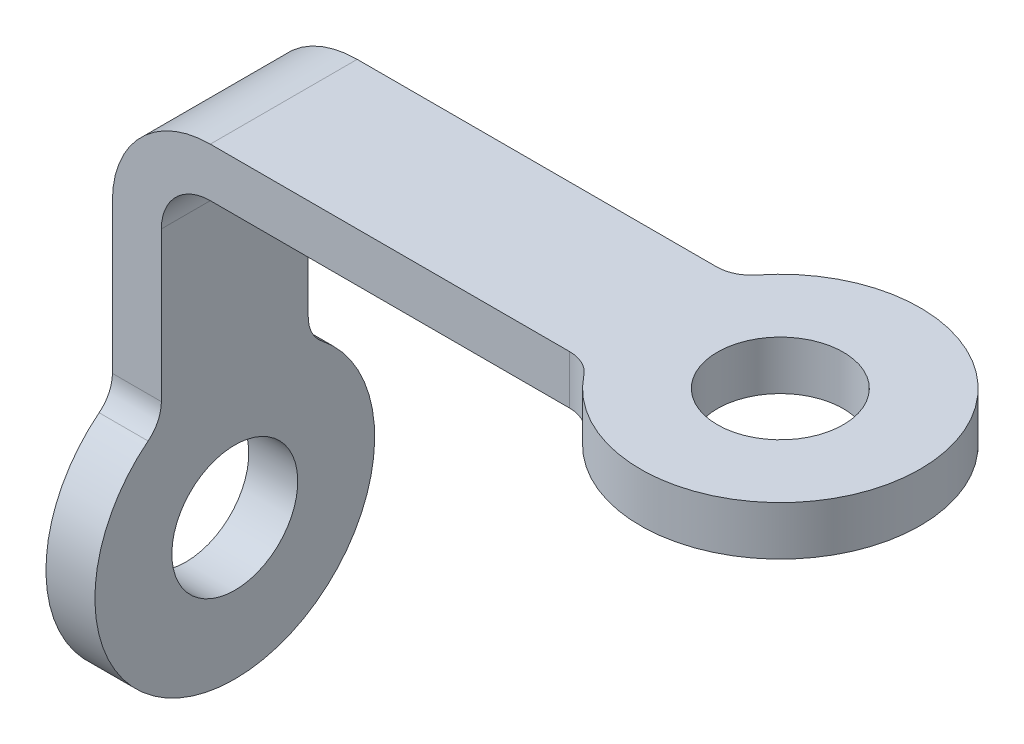
ISO-10303-21;
HEADER;
FILE_DESCRIPTION(('STEP AP214'),'2;1');
FILE_NAME('part.step','',(''),(''),'','','');
FILE_SCHEMA(('AUTOMOTIVE_DESIGN { 1 0 10303 214 1 1 1 1 }'));
ENDSEC;
DATA;
#1=APPLICATION_CONTEXT('core data for automotive mechanical design processes');
#2=APPLICATION_PROTOCOL_DEFINITION('international standard','automotive_design',2000,#1);
#3=PRODUCT_CONTEXT('',#1,'mechanical');
#4=PRODUCT('Part','Part','',(#3));
#5=PRODUCT_RELATED_PRODUCT_CATEGORY('part','',(#4));
#6=PRODUCT_DEFINITION_FORMATION('','',#4);
#7=PRODUCT_DEFINITION_CONTEXT('part definition',#1,'design');
#8=PRODUCT_DEFINITION('design','',#6,#7);
#9=PRODUCT_DEFINITION_SHAPE('','',#8);
#10=(LENGTH_UNIT() NAMED_UNIT(*) SI_UNIT(.MILLI.,.METRE.));
#11=(NAMED_UNIT(*) PLANE_ANGLE_UNIT() SI_UNIT($,.RADIAN.));
#12=(NAMED_UNIT(*) SI_UNIT($,.STERADIAN.) SOLID_ANGLE_UNIT());
#13=UNCERTAINTY_MEASURE_WITH_UNIT(LENGTH_MEASURE(1.E-05),#10,'distance_accuracy_value','');
#14=(GEOMETRIC_REPRESENTATION_CONTEXT(3) GLOBAL_UNCERTAINTY_ASSIGNED_CONTEXT((#13)) GLOBAL_UNIT_ASSIGNED_CONTEXT((#10,
#11,#12)) REPRESENTATION_CONTEXT('',''));
#15=CARTESIAN_POINT('',(0.,0.,0.));
#16=DIRECTION('',(0.,0.,1.));
#17=DIRECTION('',(1.,0.,0.));
#18=AXIS2_PLACEMENT_3D('',#15,#16,#17);
#19=CARTESIAN_POINT('',(85.,0.,10.5));
#20=DIRECTION('',(0.,-1.,0.));
#21=DIRECTION('',(0.,0.,-1.));
#22=AXIS2_PLACEMENT_3D('',#19,#20,#21);
#23=PLANE('',#22);
#24=CARTESIAN_POINT('',(85.,0.,0.));
#25=DIRECTION('',(0.,1.,0.));
#26=DIRECTION('',(0.,0.,1.));
#27=AXIS2_PLACEMENT_3D('',#24,#25,#26);
#28=CIRCLE('',#27,9.);
#29=CARTESIAN_POINT('',(85.,0.,9.));
#30=VERTEX_POINT('',#29);
#31=EDGE_CURVE('E253',#30,#30,#28,.T.);
#32=ORIENTED_EDGE('',*,*,#31,.F.);
#33=EDGE_LOOP('',(#32));
#34=FACE_BOUND('',#33,.T.);
#35=CARTESIAN_POINT('',(85.,0.,0.));
#36=DIRECTION('',(0.,1.,0.));
#37=DIRECTION('',(0.,0.,1.));
#38=AXIS2_PLACEMENT_3D('',#35,#36,#37);
#39=CIRCLE('',#38,20.);
#40=CARTESIAN_POINT('',(69.3079638032536,0.,12.4));
#41=VERTEX_POINT('',#40);
#42=CARTESIAN_POINT('',(69.3079638032536,0.,-12.4));
#43=VERTEX_POINT('',#42);
#44=EDGE_CURVE('E234',#41,#43,#39,.T.);
#45=ORIENTED_EDGE('',*,*,#44,.T.);
#46=CARTESIAN_POINT('',(65.384954754067,0.,-15.5));
#47=DIRECTION('',(0.,-1.,0.));
#48=DIRECTION('',(0.,0.,-1.));
#49=AXIS2_PLACEMENT_3D('',#46,#47,#48);
#50=CIRCLE('',#49,5.);
#51=CARTESIAN_POINT('',(65.384954754067,0.,-10.5));
#52=VERTEX_POINT('',#51);
#53=EDGE_CURVE('E230',#43,#52,#50,.T.);
#54=ORIENTED_EDGE('',*,*,#53,.T.);
#55=DIRECTION('',(-1.,0.,0.));
#56=VECTOR('',#55,1.);
#57=CARTESIAN_POINT('',(85.,0.,-10.5));
#58=LINE('',#57,#56);
#59=CARTESIAN_POINT('',(14.,0.,-10.5));
#60=VERTEX_POINT('',#59);
#61=EDGE_CURVE('E179',#52,#60,#58,.T.);
#62=ORIENTED_EDGE('',*,*,#61,.T.);
#63=DIRECTION('',(0.,0.,-1.));
#64=VECTOR('',#63,1.);
#65=CARTESIAN_POINT('',(14.,0.,10.5));
#66=LINE('',#65,#64);
#67=CARTESIAN_POINT('',(14.,0.,10.5));
#68=VERTEX_POINT('',#67);
#69=EDGE_CURVE('E159',#60,#68,#66,.F.);
#70=ORIENTED_EDGE('',*,*,#69,.T.);
#71=DIRECTION('',(-1.,0.,0.));
#72=VECTOR('',#71,1.);
#73=CARTESIAN_POINT('',(85.,0.,10.5));
#74=LINE('',#73,#72);
#75=CARTESIAN_POINT('',(65.384954754067,0.,10.5));
#76=VERTEX_POINT('',#75);
#77=EDGE_CURVE('E189',#76,#68,#74,.T.);
#78=ORIENTED_EDGE('',*,*,#77,.F.);
#79=CARTESIAN_POINT('',(65.384954754067,0.,15.5));
#80=DIRECTION('',(0.,-1.,0.));
#81=DIRECTION('',(0.,0.,-1.));
#82=AXIS2_PLACEMENT_3D('',#79,#80,#81);
#83=CIRCLE('',#82,5.);
#84=EDGE_CURVE('E69',#76,#41,#83,.T.);
#85=ORIENTED_EDGE('',*,*,#84,.T.);
#86=EDGE_LOOP('',(#45,#54,#62,#70,#78,#85));
#87=FACE_BOUND('',#86,.T.);
#88=ADVANCED_FACE('F65',(#34,#87),#23,.F.);
#89=CARTESIAN_POINT('',(0.,0.,10.5));
#90=DIRECTION('',(1.,0.,0.));
#91=DIRECTION('',(0.,1.,0.));
#92=AXIS2_PLACEMENT_3D('',#89,#90,#91);
#93=PLANE('',#92);
#94=DIRECTION('',(0.,-1.,0.));
#95=VECTOR('',#94,1.);
#96=CARTESIAN_POINT('',(0.,0.,10.5));
#97=LINE('',#96,#95);
#98=CARTESIAN_POINT('',(0.,-14.,10.5));
#99=VERTEX_POINT('',#98);
#100=CARTESIAN_POINT('',(0.,-35.384954754067,10.5));
#101=VERTEX_POINT('',#100);
#102=EDGE_CURVE('E171',#99,#101,#97,.T.);
#103=ORIENTED_EDGE('',*,*,#102,.F.);
#104=DIRECTION('',(0.,0.,-1.));
#105=VECTOR('',#104,1.);
#106=CARTESIAN_POINT('',(0.,-14.,10.5));
#107=LINE('',#106,#105);
#108=CARTESIAN_POINT('',(0.,-14.,-10.5));
#109=VERTEX_POINT('',#108);
#110=EDGE_CURVE('E160',#99,#109,#107,.T.);
#111=ORIENTED_EDGE('',*,*,#110,.T.);
#112=DIRECTION('',(0.,-1.,0.));
#113=VECTOR('',#112,1.);
#114=CARTESIAN_POINT('',(0.,0.,-10.5));
#115=LINE('',#114,#113);
#116=CARTESIAN_POINT('',(0.,-35.384954754067,-10.5));
#117=VERTEX_POINT('',#116);
#118=EDGE_CURVE('E169',#109,#117,#115,.T.);
#119=ORIENTED_EDGE('',*,*,#118,.T.);
#120=CARTESIAN_POINT('',(0.,-35.384954754067,-15.5));
#121=DIRECTION('',(1.,0.,0.));
#122=DIRECTION('',(0.,1.,0.));
#123=AXIS2_PLACEMENT_3D('',#120,#121,#122);
#124=CIRCLE('',#123,5.);
#125=CARTESIAN_POINT('',(0.,-39.3079638032536,-12.4));
#126=VERTEX_POINT('',#125);
#127=EDGE_CURVE('E223',#117,#126,#124,.T.);
#128=ORIENTED_EDGE('',*,*,#127,.T.);
#129=CARTESIAN_POINT('',(0.,-55.,0.));
#130=DIRECTION('',(-1.,0.,0.));
#131=DIRECTION('',(0.,-1.,0.));
#132=AXIS2_PLACEMENT_3D('',#129,#130,#131);
#133=CIRCLE('',#132,20.);
#134=CARTESIAN_POINT('',(0.,-39.3079638032536,12.4));
#135=VERTEX_POINT('',#134);
#136=EDGE_CURVE('E263',#126,#135,#133,.T.);
#137=ORIENTED_EDGE('',*,*,#136,.T.);
#138=CARTESIAN_POINT('',(0.,-35.384954754067,15.5));
#139=DIRECTION('',(1.,0.,0.));
#140=DIRECTION('',(0.,1.,0.));
#141=AXIS2_PLACEMENT_3D('',#138,#139,#140);
#142=CIRCLE('',#141,5.);
#143=EDGE_CURVE('E222',#135,#101,#142,.T.);
#144=ORIENTED_EDGE('',*,*,#143,.T.);
#145=EDGE_LOOP('',(#103,#111,#119,#128,#137,#144));
#146=FACE_BOUND('',#145,.T.);
#147=CARTESIAN_POINT('',(0.,-55.,0.));
#148=DIRECTION('',(-1.,0.,0.));
#149=DIRECTION('',(0.,-1.,0.));
#150=AXIS2_PLACEMENT_3D('',#147,#148,#149);
#151=CIRCLE('',#150,9.);
#152=CARTESIAN_POINT('',(0.,-64.,0.));
#153=VERTEX_POINT('',#152);
#154=EDGE_CURVE('E270',#153,#153,#151,.T.);
#155=ORIENTED_EDGE('',*,*,#154,.F.);
#156=EDGE_LOOP('',(#155));
#157=FACE_BOUND('',#156,.T.);
#158=ADVANCED_FACE('F170',(#146,#157),#93,.F.);
#159=CARTESIAN_POINT('',(7.00000000000001,-55.,10.5));
#160=DIRECTION('',(-1.,0.,0.));
#161=DIRECTION('',(0.,0.,1.));
#162=AXIS2_PLACEMENT_3D('',#159,#160,#161);
#163=PLANE('',#162);
#164=CARTESIAN_POINT('',(7.00000000000001,-55.,0.));
#165=DIRECTION('',(-1.,0.,0.));
#166=DIRECTION('',(0.,-1.,0.));
#167=AXIS2_PLACEMENT_3D('',#164,#165,#166);
#168=CIRCLE('',#167,9.);
#169=CARTESIAN_POINT('',(7.00000000000001,-64.,0.));
#170=VERTEX_POINT('',#169);
#171=EDGE_CURVE('E262',#170,#170,#168,.T.);
#172=ORIENTED_EDGE('',*,*,#171,.T.);
#173=EDGE_LOOP('',(#172));
#174=FACE_BOUND('',#173,.T.);
#175=CARTESIAN_POINT('',(7.00000000000001,-55.,0.));
#176=DIRECTION('',(-1.,0.,0.));
#177=DIRECTION('',(0.,-1.,0.));
#178=AXIS2_PLACEMENT_3D('',#175,#176,#177);
#179=CIRCLE('',#178,20.);
#180=CARTESIAN_POINT('',(7.00000000000001,-39.3079638032536,-12.4));
#181=VERTEX_POINT('',#180);
#182=CARTESIAN_POINT('',(7.00000000000001,-39.3079638032536,12.4));
#183=VERTEX_POINT('',#182);
#184=EDGE_CURVE('E259',#181,#183,#179,.T.);
#185=ORIENTED_EDGE('',*,*,#184,.F.);
#186=CARTESIAN_POINT('',(7.00000000000001,-35.384954754067,-15.5));
#187=DIRECTION('',(-1.,0.,0.));
#188=DIRECTION('',(0.,0.,1.));
#189=AXIS2_PLACEMENT_3D('',#186,#187,#188);
#190=CIRCLE('',#189,5.);
#191=CARTESIAN_POINT('',(7.00000000000001,-35.384954754067,-10.5));
#192=VERTEX_POINT('',#191);
#193=EDGE_CURVE('E221',#181,#192,#190,.T.);
#194=ORIENTED_EDGE('',*,*,#193,.T.);
#195=DIRECTION('',(0.,1.,0.));
#196=VECTOR('',#195,1.);
#197=CARTESIAN_POINT('',(7.00000000000001,-55.,-10.5));
#198=LINE('',#197,#196);
#199=CARTESIAN_POINT('',(7.00000000000001,-14.,-10.5));
#200=VERTEX_POINT('',#199);
#201=EDGE_CURVE('E177',#192,#200,#198,.T.);
#202=ORIENTED_EDGE('',*,*,#201,.T.);
#203=DIRECTION('',(0.,0.,-1.));
#204=VECTOR('',#203,1.);
#205=CARTESIAN_POINT('',(7.00000000000001,-14.,10.5));
#206=LINE('',#205,#204);
#207=CARTESIAN_POINT('',(7.00000000000001,-14.,10.5));
#208=VERTEX_POINT('',#207);
#209=EDGE_CURVE('E198',#200,#208,#206,.F.);
#210=ORIENTED_EDGE('',*,*,#209,.T.);
#211=DIRECTION('',(0.,1.,0.));
#212=VECTOR('',#211,1.);
#213=CARTESIAN_POINT('',(7.00000000000001,-55.,10.5));
#214=LINE('',#213,#212);
#215=CARTESIAN_POINT('',(7.00000000000001,-35.384954754067,10.5));
#216=VERTEX_POINT('',#215);
#217=EDGE_CURVE('E248',#216,#208,#214,.T.);
#218=ORIENTED_EDGE('',*,*,#217,.F.);
#219=CARTESIAN_POINT('',(7.00000000000001,-35.384954754067,15.5));
#220=DIRECTION('',(-1.,0.,0.));
#221=DIRECTION('',(0.,0.,1.));
#222=AXIS2_PLACEMENT_3D('',#219,#220,#221);
#223=CIRCLE('',#222,5.);
#224=EDGE_CURVE('E227',#216,#183,#223,.T.);
#225=ORIENTED_EDGE('',*,*,#224,.T.);
#226=EDGE_LOOP('',(#185,#194,#202,#210,#218,#225));
#227=FACE_BOUND('',#226,.T.);
#228=ADVANCED_FACE('F271',(#174,#227),#163,.F.);
#229=CARTESIAN_POINT('',(7.00000000000001,-7.,10.5));
#230=DIRECTION('',(0.,1.,0.));
#231=DIRECTION('',(0.,0.,1.));
#232=AXIS2_PLACEMENT_3D('',#229,#230,#231);
#233=PLANE('',#232);
#234=CARTESIAN_POINT('',(85.,-7.,0.));
#235=DIRECTION('',(0.,1.,0.));
#236=DIRECTION('',(0.,0.,1.));
#237=AXIS2_PLACEMENT_3D('',#234,#235,#236);
#238=CIRCLE('',#237,9.);
#239=CARTESIAN_POINT('',(85.,-7.,9.));
#240=VERTEX_POINT('',#239);
#241=EDGE_CURVE('E237',#240,#240,#238,.T.);
#242=ORIENTED_EDGE('',*,*,#241,.T.);
#243=EDGE_LOOP('',(#242));
#244=FACE_BOUND('',#243,.T.);
#245=DIRECTION('',(1.,0.,0.));
#246=VECTOR('',#245,1.);
#247=CARTESIAN_POINT('',(7.00000000000001,-7.,10.5));
#248=LINE('',#247,#246);
#249=CARTESIAN_POINT('',(14.,-7.,10.5));
#250=VERTEX_POINT('',#249);
#251=CARTESIAN_POINT('',(65.384954754067,-7.,10.5));
#252=VERTEX_POINT('',#251);
#253=EDGE_CURVE('E175',#250,#252,#248,.T.);
#254=ORIENTED_EDGE('',*,*,#253,.F.);
#255=DIRECTION('',(0.,0.,-1.));
#256=VECTOR('',#255,1.);
#257=CARTESIAN_POINT('',(14.,-7.,-10.5));
#258=LINE('',#257,#256);
#259=CARTESIAN_POINT('',(14.,-7.,-10.5));
#260=VERTEX_POINT('',#259);
#261=EDGE_CURVE('E194',#250,#260,#258,.T.);
#262=ORIENTED_EDGE('',*,*,#261,.T.);
#263=DIRECTION('',(1.,0.,0.));
#264=VECTOR('',#263,1.);
#265=CARTESIAN_POINT('',(7.00000000000001,-7.,-10.5));
#266=LINE('',#265,#264);
#267=CARTESIAN_POINT('',(65.384954754067,-7.,-10.5));
#268=VERTEX_POINT('',#267);
#269=EDGE_CURVE('E185',#260,#268,#266,.T.);
#270=ORIENTED_EDGE('',*,*,#269,.T.);
#271=CARTESIAN_POINT('',(65.384954754067,-7.,-15.5));
#272=DIRECTION('',(0.,1.,0.));
#273=DIRECTION('',(0.,0.,1.));
#274=AXIS2_PLACEMENT_3D('',#271,#272,#273);
#275=CIRCLE('',#274,5.);
#276=CARTESIAN_POINT('',(69.3079638032536,-7.,-12.4));
#277=VERTEX_POINT('',#276);
#278=EDGE_CURVE('E80',#268,#277,#275,.T.);
#279=ORIENTED_EDGE('',*,*,#278,.T.);
#280=CARTESIAN_POINT('',(85.,-7.,0.));
#281=DIRECTION('',(0.,1.,0.));
#282=DIRECTION('',(0.,0.,1.));
#283=AXIS2_PLACEMENT_3D('',#280,#281,#282);
#284=CIRCLE('',#283,20.);
#285=CARTESIAN_POINT('',(69.3079638032536,-7.,12.4));
#286=VERTEX_POINT('',#285);
#287=EDGE_CURVE('E183',#286,#277,#284,.T.);
#288=ORIENTED_EDGE('',*,*,#287,.F.);
#289=CARTESIAN_POINT('',(65.384954754067,-7.,15.5));
#290=DIRECTION('',(0.,1.,0.));
#291=DIRECTION('',(0.,0.,1.));
#292=AXIS2_PLACEMENT_3D('',#289,#290,#291);
#293=CIRCLE('',#292,5.);
#294=EDGE_CURVE('E12',#286,#252,#293,.T.);
#295=ORIENTED_EDGE('',*,*,#294,.T.);
#296=EDGE_LOOP('',(#254,#262,#270,#279,#288,#295));
#297=FACE_BOUND('',#296,.T.);
#298=ADVANCED_FACE('F242',(#244,#297),#233,.F.);
#299=CARTESIAN_POINT('',(0.,0.,10.5));
#300=DIRECTION('',(0.,0.,1.));
#301=DIRECTION('',(1.,0.,0.));
#302=AXIS2_PLACEMENT_3D('',#299,#300,#301);
#303=PLANE('',#302);
#304=ORIENTED_EDGE('',*,*,#102,.T.);
#305=DIRECTION('',(1.,0.,0.));
#306=VECTOR('',#305,1.);
#307=CARTESIAN_POINT('',(7.00000000000001,-35.384954754067,10.5));
#308=LINE('',#307,#306);
#309=EDGE_CURVE('E213',#101,#216,#308,.T.);
#310=ORIENTED_EDGE('',*,*,#309,.T.);
#311=ORIENTED_EDGE('',*,*,#217,.T.);
#312=CARTESIAN_POINT('',(14.,-14.,10.5));
#313=DIRECTION('',(0.,0.,1.));
#314=DIRECTION('',(1.,0.,0.));
#315=AXIS2_PLACEMENT_3D('',#312,#313,#314);
#316=CIRCLE('',#315,7.);
#317=EDGE_CURVE('E205',#208,#250,#316,.F.);
#318=ORIENTED_EDGE('',*,*,#317,.T.);
#319=ORIENTED_EDGE('',*,*,#253,.T.);
#320=DIRECTION('',(0.,-1.,0.));
#321=VECTOR('',#320,1.);
#322=CARTESIAN_POINT('',(65.384954754067,0.,10.5));
#323=LINE('',#322,#321);
#324=EDGE_CURVE('E215',#252,#76,#323,.F.);
#325=ORIENTED_EDGE('',*,*,#324,.T.);
#326=ORIENTED_EDGE('',*,*,#77,.T.);
#327=CARTESIAN_POINT('',(14.,-14.,10.5));
#328=DIRECTION('',(0.,0.,1.));
#329=DIRECTION('',(1.,0.,0.));
#330=AXIS2_PLACEMENT_3D('',#327,#328,#329);
#331=CIRCLE('',#330,14.);
#332=EDGE_CURVE('E192',#68,#99,#331,.T.);
#333=ORIENTED_EDGE('',*,*,#332,.T.);
#334=EDGE_LOOP('',(#304,#310,#311,#318,#319,#325,#326,#333));
#335=FACE_BOUND('',#334,.T.);
#336=ADVANCED_FACE('F250',(#335),#303,.T.);
#337=CARTESIAN_POINT('',(0.,0.,-10.5));
#338=DIRECTION('',(0.,0.,1.));
#339=DIRECTION('',(1.,0.,0.));
#340=AXIS2_PLACEMENT_3D('',#337,#338,#339);
#341=PLANE('',#340);
#342=ORIENTED_EDGE('',*,*,#201,.F.);
#343=DIRECTION('',(-1.,0.,0.));
#344=VECTOR('',#343,1.);
#345=CARTESIAN_POINT('',(0.,-35.384954754067,-10.5));
#346=LINE('',#345,#344);
#347=EDGE_CURVE('E178',#192,#117,#346,.T.);
#348=ORIENTED_EDGE('',*,*,#347,.T.);
#349=ORIENTED_EDGE('',*,*,#118,.F.);
#350=CARTESIAN_POINT('',(14.,-14.,-10.5));
#351=DIRECTION('',(0.,0.,1.));
#352=DIRECTION('',(1.,0.,0.));
#353=AXIS2_PLACEMENT_3D('',#350,#351,#352);
#354=CIRCLE('',#353,14.);
#355=EDGE_CURVE('E151',#109,#60,#354,.F.);
#356=ORIENTED_EDGE('',*,*,#355,.T.);
#357=ORIENTED_EDGE('',*,*,#61,.F.);
#358=DIRECTION('',(0.,1.,0.));
#359=VECTOR('',#358,1.);
#360=CARTESIAN_POINT('',(65.384954754067,0.,-10.5));
#361=LINE('',#360,#359);
#362=EDGE_CURVE('E204',#52,#268,#361,.F.);
#363=ORIENTED_EDGE('',*,*,#362,.T.);
#364=ORIENTED_EDGE('',*,*,#269,.F.);
#365=CARTESIAN_POINT('',(14.,-14.,-10.5));
#366=DIRECTION('',(0.,0.,1.));
#367=DIRECTION('',(1.,0.,0.));
#368=AXIS2_PLACEMENT_3D('',#365,#366,#367);
#369=CIRCLE('',#368,7.);
#370=EDGE_CURVE('E197',#260,#200,#369,.T.);
#371=ORIENTED_EDGE('',*,*,#370,.T.);
#372=EDGE_LOOP('',(#342,#348,#349,#356,#357,#363,#364,#371));
#373=FACE_BOUND('',#372,.T.);
#374=ADVANCED_FACE('F176',(#373),#341,.F.);
#375=CARTESIAN_POINT('',(85.,-7.,0.));
#376=DIRECTION('',(0.,1.,0.));
#377=DIRECTION('',(0.,0.,1.));
#378=AXIS2_PLACEMENT_3D('',#375,#376,#377);
#379=CYLINDRICAL_SURFACE('',#378,20.);
#380=ORIENTED_EDGE('',*,*,#287,.T.);
#381=DIRECTION('',(0.,1.,0.));
#382=VECTOR('',#381,1.);
#383=CARTESIAN_POINT('',(69.3079638032536,-7.,-12.4));
#384=LINE('',#383,#382);
#385=EDGE_CURVE('E216',#277,#43,#384,.T.);
#386=ORIENTED_EDGE('',*,*,#385,.T.);
#387=ORIENTED_EDGE('',*,*,#44,.F.);
#388=DIRECTION('',(0.,1.,0.));
#389=VECTOR('',#388,1.);
#390=CARTESIAN_POINT('',(69.3079638032536,-7.,12.4));
#391=LINE('',#390,#389);
#392=EDGE_CURVE('E81',#41,#286,#391,.F.);
#393=ORIENTED_EDGE('',*,*,#392,.T.);
#394=EDGE_LOOP('',(#380,#386,#387,#393));
#395=FACE_BOUND('',#394,.T.);
#396=ADVANCED_FACE('F240',(#395),#379,.T.);
#397=CARTESIAN_POINT('',(85.,-7.,0.));
#398=DIRECTION('',(0.,1.,0.));
#399=DIRECTION('',(0.,0.,1.));
#400=AXIS2_PLACEMENT_3D('',#397,#398,#399);
#401=CYLINDRICAL_SURFACE('',#400,9.);
#402=ORIENTED_EDGE('',*,*,#241,.F.);
#403=EDGE_LOOP('',(#402));
#404=FACE_BOUND('',#403,.T.);
#405=ORIENTED_EDGE('',*,*,#31,.T.);
#406=EDGE_LOOP('',(#405));
#407=FACE_BOUND('',#406,.T.);
#408=ADVANCED_FACE('F278',(#404,#407),#401,.F.);
#409=CARTESIAN_POINT('',(7.00000000000001,-55.,0.));
#410=DIRECTION('',(-1.,0.,0.));
#411=DIRECTION('',(0.,-1.,0.));
#412=AXIS2_PLACEMENT_3D('',#409,#410,#411);
#413=CYLINDRICAL_SURFACE('',#412,9.);
#414=ORIENTED_EDGE('',*,*,#171,.F.);
#415=EDGE_LOOP('',(#414));
#416=FACE_BOUND('',#415,.T.);
#417=ORIENTED_EDGE('',*,*,#154,.T.);
#418=EDGE_LOOP('',(#417));
#419=FACE_BOUND('',#418,.T.);
#420=ADVANCED_FACE('F277',(#416,#419),#413,.F.);
#421=CARTESIAN_POINT('',(7.00000000000001,-55.,0.));
#422=DIRECTION('',(-1.,0.,0.));
#423=DIRECTION('',(0.,-1.,0.));
#424=AXIS2_PLACEMENT_3D('',#421,#422,#423);
#425=CYLINDRICAL_SURFACE('',#424,20.);
#426=ORIENTED_EDGE('',*,*,#136,.F.);
#427=DIRECTION('',(-1.,0.,0.));
#428=VECTOR('',#427,1.);
#429=CARTESIAN_POINT('',(7.00000000000001,-39.3079638032536,-12.4));
#430=LINE('',#429,#428);
#431=EDGE_CURVE('E208',#126,#181,#430,.F.);
#432=ORIENTED_EDGE('',*,*,#431,.T.);
#433=ORIENTED_EDGE('',*,*,#184,.T.);
#434=DIRECTION('',(-1.,0.,0.));
#435=VECTOR('',#434,1.);
#436=CARTESIAN_POINT('',(7.00000000000001,-39.3079638032536,12.4));
#437=LINE('',#436,#435);
#438=EDGE_CURVE('E210',#183,#135,#437,.T.);
#439=ORIENTED_EDGE('',*,*,#438,.T.);
#440=EDGE_LOOP('',(#426,#432,#433,#439));
#441=FACE_BOUND('',#440,.T.);
#442=ADVANCED_FACE('F276',(#441),#425,.T.);
#443=CARTESIAN_POINT('',(14.,-14.,10.5));
#444=DIRECTION('',(0.,0.,-1.));
#445=DIRECTION('',(-1.,0.,0.));
#446=AXIS2_PLACEMENT_3D('',#443,#444,#445);
#447=CYLINDRICAL_SURFACE('',#446,14.);
#448=ORIENTED_EDGE('',*,*,#332,.F.);
#449=ORIENTED_EDGE('',*,*,#69,.F.);
#450=ORIENTED_EDGE('',*,*,#355,.F.);
#451=ORIENTED_EDGE('',*,*,#110,.F.);
#452=EDGE_LOOP('',(#448,#449,#450,#451));
#453=FACE_BOUND('',#452,.T.);
#454=ADVANCED_FACE('F158',(#453),#447,.T.);
#455=CARTESIAN_POINT('',(14.,-14.,10.5));
#456=DIRECTION('',(0.,0.,1.));
#457=DIRECTION('',(1.,0.,0.));
#458=AXIS2_PLACEMENT_3D('',#455,#456,#457);
#459=CYLINDRICAL_SURFACE('',#458,7.);
#460=ORIENTED_EDGE('',*,*,#317,.F.);
#461=ORIENTED_EDGE('',*,*,#209,.F.);
#462=ORIENTED_EDGE('',*,*,#370,.F.);
#463=ORIENTED_EDGE('',*,*,#261,.F.);
#464=EDGE_LOOP('',(#460,#461,#462,#463));
#465=FACE_BOUND('',#464,.T.);
#466=ADVANCED_FACE('F298',(#465),#459,.F.);
#467=CARTESIAN_POINT('',(7.,-35.384954754067,-15.5));
#468=DIRECTION('',(-1.,0.,0.));
#469=DIRECTION('',(0.,-1.,0.));
#470=AXIS2_PLACEMENT_3D('',#467,#468,#469);
#471=CYLINDRICAL_SURFACE('',#470,5.);
#472=ORIENTED_EDGE('',*,*,#193,.F.);
#473=ORIENTED_EDGE('',*,*,#431,.F.);
#474=ORIENTED_EDGE('',*,*,#127,.F.);
#475=ORIENTED_EDGE('',*,*,#347,.F.);
#476=EDGE_LOOP('',(#472,#473,#474,#475));
#477=FACE_BOUND('',#476,.T.);
#478=ADVANCED_FACE('F299',(#477),#471,.F.);
#479=CARTESIAN_POINT('',(7.,-35.384954754067,15.5));
#480=DIRECTION('',(-1.,0.,0.));
#481=DIRECTION('',(0.,-1.,0.));
#482=AXIS2_PLACEMENT_3D('',#479,#480,#481);
#483=CYLINDRICAL_SURFACE('',#482,5.);
#484=ORIENTED_EDGE('',*,*,#224,.F.);
#485=ORIENTED_EDGE('',*,*,#309,.F.);
#486=ORIENTED_EDGE('',*,*,#143,.F.);
#487=ORIENTED_EDGE('',*,*,#438,.F.);
#488=EDGE_LOOP('',(#484,#485,#486,#487));
#489=FACE_BOUND('',#488,.T.);
#490=ADVANCED_FACE('F303',(#489),#483,.F.);
#491=CARTESIAN_POINT('',(65.384954754067,-7.,-15.5));
#492=DIRECTION('',(0.,1.,0.));
#493=DIRECTION('',(0.,0.,1.));
#494=AXIS2_PLACEMENT_3D('',#491,#492,#493);
#495=CYLINDRICAL_SURFACE('',#494,5.);
#496=ORIENTED_EDGE('',*,*,#278,.F.);
#497=ORIENTED_EDGE('',*,*,#362,.F.);
#498=ORIENTED_EDGE('',*,*,#53,.F.);
#499=ORIENTED_EDGE('',*,*,#385,.F.);
#500=EDGE_LOOP('',(#496,#497,#498,#499));
#501=FACE_BOUND('',#500,.T.);
#502=ADVANCED_FACE('F306',(#501),#495,.F.);
#503=CARTESIAN_POINT('',(65.384954754067,-7.,15.5));
#504=DIRECTION('',(0.,1.,0.));
#505=DIRECTION('',(0.,0.,1.));
#506=AXIS2_PLACEMENT_3D('',#503,#504,#505);
#507=CYLINDRICAL_SURFACE('',#506,5.);
#508=ORIENTED_EDGE('',*,*,#294,.F.);
#509=ORIENTED_EDGE('',*,*,#392,.F.);
#510=ORIENTED_EDGE('',*,*,#84,.F.);
#511=ORIENTED_EDGE('',*,*,#324,.F.);
#512=EDGE_LOOP('',(#508,#509,#510,#511));
#513=FACE_BOUND('',#512,.T.);
#514=ADVANCED_FACE('F61',(#513),#507,.F.);
#515=CLOSED_SHELL('',(#88,#158,#228,#298,#336,#374,#396,#408,#420,#442,#454,#466,#478,#490,#502,#514));
#516=MANIFOLD_SOLID_BREP('B2',#515);
#517=ADVANCED_BREP_SHAPE_REPRESENTATION('',(#18,#516),#14);
#518=SHAPE_DEFINITION_REPRESENTATION(#9,#517);
ENDSEC;
END-ISO-10303-21;
